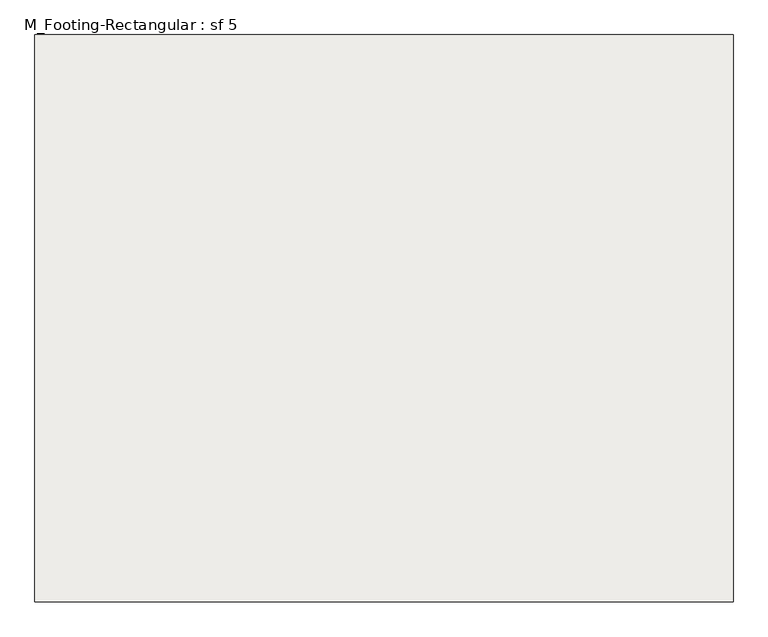
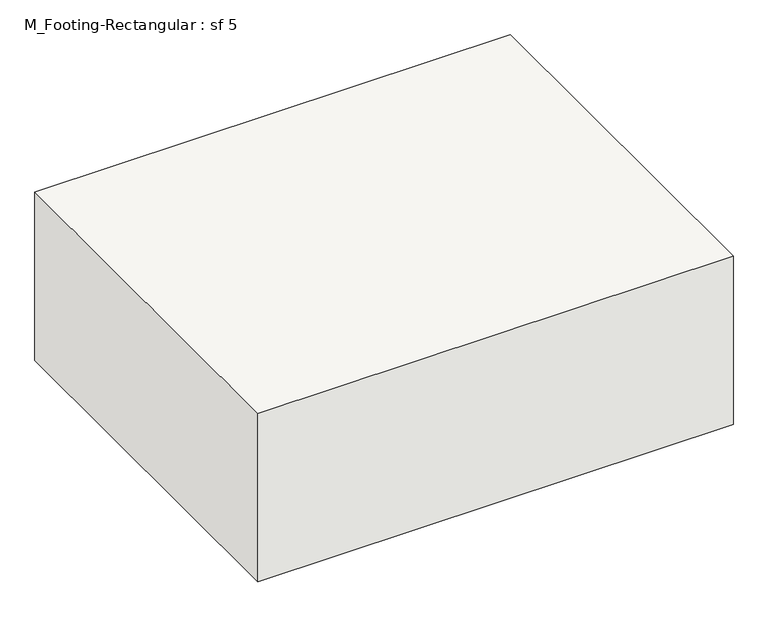
"""IFC4 building model written with IfcOpenShell, lengths in millimetres: slab geometry, M_Footing-Rectangular : sf 5."""

from ifc_helpers import new_model, si_unit, frame, origin, place, context, project, spatial, polyline, outline, extrude, source, transform, mapped, element, save


def m_footing_rectangular_sf_5_e6d23758(model_context):
    return source(origin(), model_context, "Body", "SweptSolid", [
        extrude(outline(polyline([(609.6, 495.3), (609.6, -495.3), (-609.6, -495.3), (-609.6, 495.3), (609.6, 495.3)])), frame((0.0, 0.0, -457.2), z_axis=(0.0, 0.0, 1.0), x_axis=(1.0, 0.0, 0.0)), (0.0, 0.0, 1.0), 457.2),
    ])


if __name__ == "__main__":
    model = new_model("IFC4")
    model_context = context("Model", 3, world=origin())
    ifc_project = project(units=[si_unit("LENGTHUNIT", "METRE", prefix="MILLI")], contexts=[model_context])
    site = spatial("IfcSite", under=ifc_project)
    building = spatial("IfcBuilding", under=site)
    placement = place(None, origin())
    m_footing_rectangular_sf_5_shape = m_footing_rectangular_sf_5_e6d23758(model_context)
    element("IfcSlab", 1, ObjectType="M_Footing-Rectangular : sf 5", at=placement, inside=building, context=model_context, shape_type="MappedRepresentation", body=[
        mapped(m_footing_rectangular_sf_5_shape, transform((0.0, 0.0, 0.0), x_axis=(1.0, 0.0, 0.0), y_axis=(0.0, 1.0, 0.0), z_axis=(0.0, 0.0, 1.0))),
    ])
    save(model, "model.ifc")

# Revit data of these elements
# Type "M_Footing-Rectangular : sf 5"
#   Width = 1219.2 mm
#   Length = 990.6 mm
#   Foundation Thickness = 457.2 mm
#   Structural Material [instance default] = Concrete, Cast-in-Place gray
#   Assembly Code = ""
# Element 1 (IfcSlab, "M_Footing-Rectangular : sf 5")
#   Materials on its faces: "Concrete, Cast-in-Place gray"
# Materials
#   "Concrete, Cast-in-Place gray": class "Concrete", colour RGB 192 192 192, transparency 0, Description = "Cast-in-place concrete", Cost = 0
